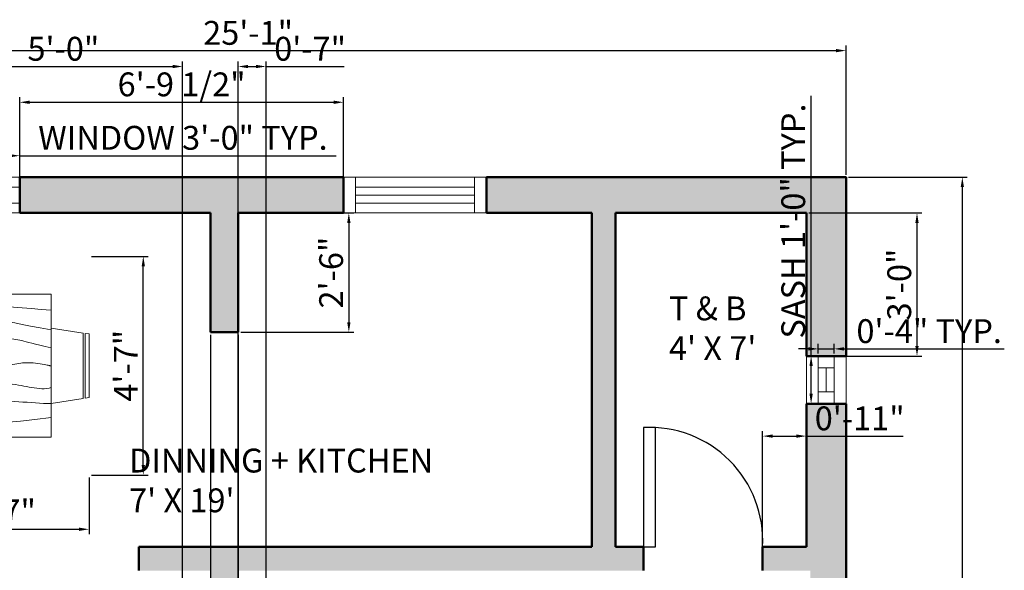
# Model space of a CAD drawing. Units: inches. Extents: x 2247 to 2697, y 1573 to 2133.
# Tile 4 of 4: x 2409 to 2657, y 1993 to 2132. Entities that reach past the tile are written whole.
import ezdxf

# ---------------------------------------------------------------- set-up
doc = ezdxf.new("R2010")
doc.units = ezdxf.units.IN
for name, color, linetype, lineweight in [('A-ANNO-DIMS', 2, 'Continuous', 18), ('A-AREA-IDEN', 7, 'Continuous', 25), ('A-DOOR', 4, 'Continuous', 25), ('A-FURN', 8, 'Continuous', 18), ('A-GLAZ', 4, 'Continuous', 18), ('A-WALL', 7, 'Continuous', 50)]:
    doc.layers.add(name, color=color, linetype=linetype, lineweight=lineweight)
doc.layers.add('A-WALL-PATT', color=67, linetype='Continuous', lineweight=13, true_color=0x727430)
doc.styles.get("Standard").update_dxf_attribs({"font": 'arial.ttf'})
doc.dimstyles.new('ISO-25', dxfattribs={"dimtxt": 6, "dimasz": 2.5, "dimexe": 1.25, "dimexo": 0.625, "dimtad": 1, "dimlunit": 3, "dimtxsty": 'Standard', "dimcen": 2.5, "dimadec": 0, "dimazin": 0, "dimtfac": 1, "dimtmove": 0, "dimatfit": 3, "dimfxl": 1, "dimarcsym": 0})

# ---------------------------------------------------------------- blocks, each defined once
blk = doc.blocks.new('*D1')
at = {"layer": 'A-ANNO-DIMS', "color": 0, "lineweight": -2, "transparency": 16777216}
for p, q in [((2316.09, 2092.98), (2316.09, 2125.46)), ((2318.59, 2124.21), (2614.59, 2124.21)), ((2617.09, 2092.98), (2617.09, 2125.46))]:
    blk.add_line(p, q, dxfattribs=at)
at = {"layer": 'A-ANNO-DIMS', "color": 0, "transparency": 16777216}
for points in [[(2318.59, 2124.63), (2318.59, 2123.79), (2316.09, 2124.21)], [(2614.59, 2124.63), (2614.59, 2123.79), (2617.09, 2124.21)]]:
    blk.add_solid(points, dxfattribs=at)
at = {"layer": 'Defpoints', "color": 0, "transparency": 16777216}
for p in [(2617.09, 2124.21), (2316.09, 2092.36), (2617.09, 2092.36)]:
    blk.add_point(p, dxfattribs=at)
at = {"layer": 'A-ANNO-DIMS', "color": 0, "transparency": 16777216, "insert": (2466.59, 2127.9), "char_height": 6, "attachment_point": 5}
blk.add_mtext('25\'-1"', dxfattribs=at)
blk = doc.blocks.new('*D2')
at = {"layer": 'A-ANNO-DIMS', "color": 0, "lineweight": -2, "transparency": 16777216}
for p, q in [((2617.72, 2092.36), (2647.6, 2092.36)), ((2646.35, 2089.86), (2646.35, 1604.86)), ((2617.72, 1602.36), (2647.6, 1602.36))]:
    blk.add_line(p, q, dxfattribs=at)
at = {"layer": 'A-ANNO-DIMS', "color": 0, "transparency": 16777216}
for points in [[(2645.94, 2089.86), (2646.77, 2089.86), (2646.35, 2092.36)], [(2645.94, 1604.86), (2646.77, 1604.86), (2646.35, 1602.36)]]:
    blk.add_solid(points, dxfattribs=at)
at = {"layer": 'Defpoints', "color": 0, "transparency": 16777216}
for p in [(2617.09, 2092.36), (2617.09, 1602.36), (2646.35, 1602.36)]:
    blk.add_point(p, dxfattribs=at)
at = {"layer": 'A-ANNO-DIMS', "color": 0, "transparency": 16777216, "insert": (2642.66, 1847.36), "char_height": 6, "attachment_point": 5, "rotation": 90}
blk.add_mtext('40\'-10"', dxfattribs=at)
blk = doc.blocks.new('Dining Set - 36 x 72 in.')
for p, q in [((-22, 27.5), (-22.1562, 26.50042)), ((-22, 27.5), (-6, 27.5)), ((-5.8437, 26.49966), (-6, 27.5)), ((6, 27.5), (5.8438, 26.50042)), ((6, 27.5), (22, 27.5)), ((22.1563, 26.49966), (22, 27.5)), ((-22.2343, 26.00059), (-23.4847, 17.99762)), ((-22.2304, 26), (-5.7608, 26)), ((-5.8416, 26.5), (-22.1534, 26.5)), ((-4.5152, 17.99762), (-5.7655, 25.99926)), ((5.7657, 26.00059), (4.5153, 17.99762)), ((5.7696, 26), (22.2392, 26)), ((22.1584, 26.5), (5.8466, 26.5)), ((23.4848, 17.99762), (22.2345, 25.99926)), ((36, 18), (-36, 18)), ((-36, 18), (-36, -18)), ((36, -18), (36, 18)), ((-45.5, 8), (-44.5004, 8.15617)), ((-45.5, 8), (-45.5, -8)), ((-44.5, -8.15843), (-44.5, 8.15338)), ((-44.0006, 8.23428), (-35.9976, 9.48474)), ((-44, 8.23041), (-44, -8.23915)), ((44.0006, 8.23428), (35.9976, 9.48474)), ((44, 8.23041), (44, -8.23915)), ((44.5, -8.15843), (44.5, 8.15338)), ((45.5, 8), (44.5005, 8.15617)), ((45.5, 8), (45.5, -8)), ((-44.4997, -8.15631), (-45.5, -8)), ((-35.9976, -9.48476), (-43.9993, -8.2345)), ((35.9976, -9.48476), (43.9993, -8.2345)), ((44.4997, -8.15631), (45.5, -8)), ((-36, -18), (36, -18)), ((-22.2343, -26.0006), (-23.4847, -17.99762)), ((-4.5152, -17.99762), (-5.7655, -25.99928)), ((5.7657, -26.0006), (4.5153, -17.99762)), ((23.4848, -17.99762), (22.2345, -25.99928)), ((-22.2304, -26), (-5.7608, -26)), ((-22, -27.5), (-22.1562, -26.50044)), ((-5.8416, -26.5), (-22.1534, -26.5)), ((-5.8437, -26.49967), (-6, -27.5)), ((5.7696, -26), (22.2392, -26)), ((6, -27.5), (5.8438, -26.50044)), ((22.1584, -26.5), (5.8466, -26.5)), ((22.1563, -26.49967), (22, -27.5)), ((-22, -27.5), (-6, -27.5)), ((6, -27.5), (22, -27.5))]:
    blk.add_line(p, q)
for points in [[(-36, 15), (-31.1772, 14.97754), (-26.8079, 14.91406), (-22.8538, 14.81543), (-19.276, 14.6875), (-16.0362, 14.53613), (-13.0957, 14.36718), (-10.4159, 14.18652), (-7.9583, 14), (-5.6904, 13.81315), (-3.6035, 13.63021), (-1.6954, 13.45508), (0.0365, 13.29166), (1.5945, 13.14388), (2.9811, 13.01562), (4.1988, 12.9108), (5.25, 12.83333), (6.1393, 12.78613), (6.8802, 12.76823), (7.4883, 12.77767), (7.9792, 12.8125), (8.3685, 12.87077), (8.6719, 12.95052), (8.9049, 13.0498), (9.0833, 13.16666), (9.2205, 13.29899), (9.3216, 13.44401), (9.3895, 13.59879), (9.4271, 13.76041), (9.4373, 13.92594), (9.4232, 14.09245), (9.3875, 14.257), (9.3333, 14.41666), (9.2638, 14.56917), (9.1836, 14.71484), (9.0975, 14.85465), (9.0104, 14.98958), (8.9272, 15.1206), (8.8529, 15.2487), (8.7922, 15.37483), (8.75, 15.5), (8.7305, 15.62467), (8.7344, 15.74739), (8.7617, 15.86621), (8.8125, 15.97916), (8.8867, 16.08431), (8.9844, 16.17968), (9.1055, 16.26334), (9.25, 16.33333), (9.4189, 16.38802), (9.6172, 16.42708), (9.8506, 16.45052), (10.125, 16.45833), (10.4463, 16.45052), (10.8203, 16.42708), (11.2529, 16.38802), (11.75, 16.33333), (12.3184, 16.26318), (12.9694, 16.17838), (13.7151, 16.07991), (14.5677, 15.96875), (15.5395, 15.84586), (16.6426, 15.71224), (17.8893, 15.56884), (19.2917, 15.41666), (20.859, 15.25667), (22.5879, 15.08984), (24.4721, 14.91715), (26.5052, 14.73958), (28.6809, 14.5581), (30.9929, 14.3737), (33.4347, 14.18733), (36, 14)], [(-36, 10), (-28.9766, 10.14274), (-23.1725, 10.20442), (-18.4241, 10.19775), (-14.5677, 10.13541), (-11.4399, 10.03011), (-8.877, 9.89453), (-6.7154, 9.74137), (-4.7917, 9.58333), (-2.9698, 9.43082), (-1.2246, 9.28515), (0.4415, 9.14534), (2.026, 9.01041), (3.5266, 8.87939), (4.9408, 8.7513), (6.266, 8.62516), (7.5, 8.5), (8.6411, 8.37549), (9.6914, 8.2539), (10.6538, 8.13818), (11.5312, 8.03125), (12.3267, 7.93603), (13.043, 7.85547), (13.6831, 7.79248), (14.25, 7.75), (14.7471, 7.7303), (15.1797, 7.73307), (15.5537, 7.75732), (15.875, 7.80208), (16.1494, 7.86637), (16.3828, 7.94922), (16.5811, 8.04964), (16.75, 8.16666), (16.8944, 8.29915), (17.0143, 8.44531), (17.1089, 8.60319), (17.1771, 8.77083), (17.218, 8.94629), (17.2305, 9.1276), (17.2137, 9.31282), (17.1667, 9.5), (17.0895, 9.6875), (16.987, 9.875), (16.8649, 10.0625), (16.7292, 10.25), (16.5856, 10.4375), (16.4401, 10.625), (16.2985, 10.8125), (16.1667, 11), (16.05, 11.18733), (15.9518, 11.3737), (15.8752, 11.5581), (15.8229, 11.73958), (15.798, 11.91715), (15.8034, 12.08984), (15.842, 12.25667), (15.9167, 12.41666), (16.0295, 12.56836), (16.1784, 12.70833), (16.3605, 12.83268), (16.5729, 12.9375), (16.8127, 13.01888), (17.0768, 13.07291), (17.3625, 13.0957), (17.6667, 13.08333), (17.9894, 13.03312), (18.3418, 12.94726), (18.7382, 12.82918), (19.1927, 12.68229), (19.7195, 12.51001), (20.3327, 12.31575), (21.0465, 12.10294), (21.875, 11.875), (22.8357, 11.63354), (23.959, 11.37304), (25.2786, 11.08618), (26.8282, 10.76562), (28.6414, 10.40405), (30.752, 9.99414), (33.1936, 9.52856), (36, 9)], [(-36, 5.5), (-30.7157, 5.3348), (-26.069, 5.20963), (-21.9946, 5.11767), (-18.4271, 5.05208), (-15.3009, 5.00602), (-12.5508, 4.97265), (-10.1112, 4.94515), (-7.9167, 4.91666), (-5.909, 4.88167), (-4.0586, 4.83984), (-2.3429, 4.79215), (-0.7396, 4.73958), (0.7739, 4.6831), (2.22, 4.6237), (3.6213, 4.56233), (5, 4.5), (6.373, 4.43782), (7.7344, 4.3776), (9.0723, 4.32129), (10.375, 4.27083), (11.6309, 4.22819), (12.8281, 4.19531), (13.9551, 4.17415), (15, 4.16666), (15.954, 4.17448), (16.819, 4.19791), (17.6001, 4.23698), (18.3021, 4.29166), (18.9299, 4.36198), (19.4883, 4.44791), (19.9823, 4.54948), (20.4167, 4.66666), (20.7969, 4.79899), (21.1302, 4.94401), (21.4245, 5.09879), (21.6875, 5.26041), (21.9271, 5.42594), (22.1511, 5.59245), (22.3672, 5.757), (22.5834, 5.91666), (22.8065, 6.06868), (23.0404, 6.21093), (23.2879, 6.34147), (23.5521, 6.45833), (23.8358, 6.55957), (24.142, 6.64323), (24.4735, 6.70735), (24.8334, 6.75), (25.2235, 6.76969), (25.642, 6.76692), (26.0858, 6.74267), (26.5521, 6.69791), (27.0379, 6.63362), (27.5404, 6.55078), (28.0565, 6.45036), (28.5834, 6.33333), (29.1242, 6.19987), (29.7071, 6.04687), (30.3661, 5.87044), (31.1354, 5.66666), (32.0493, 5.43164), (33.142, 5.16146), (34.4475, 4.85221), (36, 4.5)], [(-36, -1), (-30.7915, -0.6591), (-26.0195, -0.38216), (-21.6519, -0.16284), (-17.6563, 0.00521), (-14.0005, 0.12833), (-10.6523, 0.21289), (-7.5796, 0.26522), (-4.75, 0.29166), (-2.134, 0.29793), (0.2878, 0.28711), (2.5317, 0.26163), (4.6146, 0.22396), (6.5529, 0.17651), (8.3633, 0.12174), (10.0623, 0.06209), (11.6667, 0), (13.1899, -0.06201), (14.6341, -0.1211), (15.9982, -0.17432), (17.2813, -0.21875), (18.4823, -0.25147), (19.6003, -0.26953), (20.6343, -0.27002), (21.5834, -0.25), (22.4481, -0.20768), (23.2357, -0.14584), (23.9549, -0.06836), (24.6146, 0.02083), (25.2235, 0.11784), (25.7904, 0.21875), (26.3241, 0.31966), (26.8334, 0.41666), (27.3265, 0.50618), (27.8099, 0.58593), (28.2894, 0.65397), (28.7709, 0.70833), (29.2601, 0.74707), (29.763, 0.76823), (30.2855, 0.76985), (30.8334, 0.75), (31.4088, 0.70784), (31.9994, 0.64713), (32.589, 0.57275), (33.1615, 0.48958), (33.7008, 0.4025), (34.1908, 0.3164), (34.6153, 0.23616), (34.9584, 0.16666), (35.2099, 0.11165), (35.3848, 0.07031), (35.504, 0.04069), (35.5886, 0.02083), (35.6594, 0.00879), (35.7377, 0.0026), (35.8442, 0.00032), (36, 0)], [(-36, -6.5), (-27.1843, -6.31267), (-20.084, -6.1263), (-14.469, -5.9419), (-10.1094, -5.76042), (-6.7752, -5.58285), (-4.2363, -5.41016), (-2.2629, -5.24333), (-0.625, -5.08334), (0.8708, -4.93099), (2.2715, -4.78646), (3.5872, -4.64974), (4.8281, -4.52084), (6.0046, -4.39974), (7.127, -4.28646), (8.2053, -4.18099), (9.25, -4.08334), (10.2705, -3.99382), (11.2734, -3.91407), (12.2647, -3.84603), (13.25, -3.79167), (14.2354, -3.75293), (15.2266, -3.73177), (16.2295, -3.73015), (17.25, -3.75), (18.2912, -3.79248), (19.3451, -3.85547), (20.4009, -3.93604), (21.4479, -4.03125), (22.4754, -4.13819), (23.4727, -4.25391), (24.4289, -4.37549), (25.3334, -4.5), (26.1785, -4.62492), (26.9694, -4.74935), (27.7145, -4.87281), (28.4219, -4.99479), (29.1, -5.11483), (29.7572, -5.23242), (30.4016, -5.34709), (31.0417, -5.45834), (31.6837, -5.56437), (32.3262, -5.65821), (32.9658, -5.73153), (33.599, -5.77604), (34.2224, -5.78345), (34.8327, -5.74545), (35.4264, -5.65373), (36, -5.5)], [(-36, -10), (-26.4022, -9.81299), (-18.4675, -9.62891), (-11.9839, -9.45069), (-6.7396, -9.28125), (-2.5226, -9.12354), (0.8789, -8.98047), (3.6769, -8.85498), (6.0833, -8.75), (8.2767, -8.66765), (10.3021, -8.60677), (12.1712, -8.56543), (13.8958, -8.54167), (15.4876, -8.53353), (16.9583, -8.53907), (18.3197, -8.55632), (19.5834, -8.58334), (20.7616, -8.61841), (21.8685, -8.66081), (22.9188, -8.71004), (23.9271, -8.76563), (24.9081, -8.82707), (25.8763, -8.89388), (26.8465, -8.96558), (27.8334, -9.04167), (28.8474, -9.12118), (29.8828, -9.20117), (30.93, -9.27824), (31.9792, -9.34896), (33.0205, -9.40991), (34.0443, -9.45768), (35.0407, -9.48885), (36, -9.5)], [(-36, -14.5), (-30.0881, -14.33513), (-25.0332, -14.21224), (-20.7312, -14.12647), (-17.0781, -14.07292), (-13.97, -14.04671), (-11.3027, -14.04297), (-8.9724, -14.05681), (-6.875, -14.08334), (-4.9224, -14.11833), (-3.0905, -14.16016), (-1.3709, -14.20785), (0.2448, -14.26042), (1.7647, -14.3169), (3.1973, -14.3763), (4.5507, -14.43767), (5.8333, -14.5), (7.0554, -14.5621), (8.235, -14.62175), (9.3922, -14.67652), (10.5469, -14.72396), (11.7192, -14.76164), (12.929, -14.78711), (14.1965, -14.79794), (15.5417, -14.79167), (16.9933, -14.76424), (18.6152, -14.70508), (20.4804, -14.60197), (22.6615, -14.44271), (25.2312, -14.21509), (28.2624, -13.9069), (31.8277, -13.50594), (36, -13)]]:
    blk.add_lwpolyline(points)
blk = doc.blocks.new('DOOR-SWING-30IN')
blk.add_lwpolyline([(0, 0), (3, 0), (3, 30), (0, 30)], close=True)
blk.add_arc((1.5, 1.5), 28.54, 356.9872, 93.0128)
blk = doc.blocks.new('WIN-36IN')
for p, q in [((0, 9), (36, 9)), ((0, 6.5), (36, 6.5)), ((3, 2.5), (3, 6.5)), ((33, 2.5), (33, 6.5)), ((0, 2.5), (36, 2.5)), ((3, 4.5), (33, 4.5)), ((0, 0), (36, 0))]:
    blk.add_line(p, q)
blk = doc.blocks.new('WIN-SASH-12IN')
for p, q in [((0, 0), (0, 12)), ((4, 0), (4, 12)), ((0, 9), (4, 9)), ((2, 3), (2, 9)), ((0, 3), (4, 3))]:
    blk.add_line(p, q)
blk = doc.blocks.new('*D13')
at = {"layer": 'A-ANNO-DIMS', "color": 0, "lineweight": -2, "transparency": 16777216}
for p, q in [((2373.09, 2092.98), (2373.09, 2099.01)), ((2375.59, 2097.76), (2406.59, 2097.76)), ((2409.09, 2092.98), (2409.09, 2099.01)), ((2409.09, 2097.76), (2488.77, 2097.76))]:
    blk.add_line(p, q, dxfattribs=at)
at = {"layer": 'A-ANNO-DIMS', "color": 0, "transparency": 16777216}
for points in [[(2375.59, 2098.18), (2375.59, 2097.34), (2373.09, 2097.76)], [(2406.59, 2098.18), (2406.59, 2097.34), (2409.09, 2097.76)]]:
    blk.add_solid(points, dxfattribs=at)
at = {"layer": 'Defpoints', "color": 0, "transparency": 16777216}
for p in [(2409.09, 2097.76), (2373.09, 2092.36), (2409.09, 2092.36)]:
    blk.add_point(p, dxfattribs=at)
at = {"layer": 'A-ANNO-DIMS', "color": 0, "transparency": 16777216, "insert": (2450.18, 2101.49), "char_height": 6, "attachment_point": 5}
blk.add_mtext('WINDOW 3\'-0" TYP.', dxfattribs=at)
blk = doc.blocks.new('*D17')
at = {"layer": 'A-ANNO-DIMS', "color": 0, "lineweight": -2, "transparency": 16777216}
for p, q in [((2608.29, 2047.36), (2608.29, 2112.81)), ((2609.47, 2047.36), (2607.04, 2047.36)), ((2608.29, 2037.86), (2608.29, 2044.86)), ((2609.47, 2035.36), (2607.04, 2035.36))]:
    blk.add_line(p, q, dxfattribs=at)
at = {"layer": 'A-ANNO-DIMS', "color": 0, "transparency": 16777216}
for points in [[(2607.88, 2044.86), (2608.71, 2044.86), (2608.29, 2047.36)], [(2607.88, 2037.86), (2608.71, 2037.86), (2608.29, 2035.36)]]:
    blk.add_solid(points, dxfattribs=at)
at = {"layer": 'Defpoints', "color": 0, "transparency": 16777216}
for p in [(2608.29, 2047.36), (2610.09, 2047.36), (2610.09, 2035.36)]:
    blk.add_point(p, dxfattribs=at)
at = {"layer": 'A-ANNO-DIMS', "color": 0, "transparency": 16777216, "insert": (2604.57, 2081.33), "char_height": 6, "attachment_point": 5, "rotation": 90}
blk.add_mtext('SASH 1\'-0" TYP.', dxfattribs=at)
blk = doc.blocks.new('*D18')
at = {"layer": 'A-ANNO-DIMS', "color": 0, "lineweight": -2, "transparency": 16777216}
for p, q in [((2610.09, 2047.98), (2610.09, 2050.41)), ((2614.09, 2047.98), (2614.09, 2050.41)), ((2607.59, 2049.16), (2605.09, 2049.16)), ((2610.09, 2049.16), (2614.09, 2049.16)), ((2616.59, 2049.16), (2656.92, 2049.16))]:
    blk.add_line(p, q, dxfattribs=at)
at = {"layer": 'A-ANNO-DIMS', "color": 0, "transparency": 16777216}
for points in [[(2607.59, 2049.58), (2607.59, 2048.74), (2610.09, 2049.16)], [(2616.59, 2049.58), (2616.59, 2048.74), (2614.09, 2049.16)]]:
    blk.add_solid(points, dxfattribs=at)
at = {"layer": 'Defpoints', "color": 0, "transparency": 16777216}
for p in [(2610.09, 2047.36), (2614.09, 2049.16), (2614.09, 2047.36)]:
    blk.add_point(p, dxfattribs=at)
at = {"layer": 'A-ANNO-DIMS', "color": 0, "transparency": 16777216, "insert": (2638.01, 2052.85), "char_height": 6, "attachment_point": 5}
blk.add_mtext('0\'-4" TYP.', dxfattribs=at)
blk = doc.blocks.new('*D21')
at = {"layer": 'A-ANNO-DIMS', "color": 0, "lineweight": -2, "transparency": 16777216}
for p, q in [((2335.55, 2016.79), (2335.55, 2002.52)), ((2426.55, 2016.79), (2426.55, 2002.52)), ((2338.05, 2003.77), (2424.05, 2003.77))]:
    blk.add_line(p, q, dxfattribs=at)
at = {"layer": 'A-ANNO-DIMS', "color": 0, "transparency": 16777216}
for points in [[(2338.05, 2004.18), (2338.05, 2003.35), (2335.55, 2003.77)], [(2424.05, 2004.18), (2424.05, 2003.35), (2426.55, 2003.77)]]:
    blk.add_solid(points, dxfattribs=at)
at = {"layer": 'Defpoints', "color": 0, "transparency": 16777216}
for p in [(2335.55, 2017.42), (2426.55, 2017.42), (2426.55, 2003.77)]:
    blk.add_point(p, dxfattribs=at)
at = {"layer": 'A-ANNO-DIMS', "color": 0, "transparency": 16777216, "insert": (2381.05, 2007.49), "char_height": 6, "attachment_point": 5}
blk.add_mtext('DINING SET 7\'-7"', dxfattribs=at)
blk = doc.blocks.new('*D22')
at = {"layer": 'A-ANNO-DIMS', "color": 0, "lineweight": -2, "transparency": 16777216}
for p, q in [((2427.18, 2072.42), (2441.45, 2072.42)), ((2440.2, 2019.92), (2440.2, 2069.92)), ((2427.18, 2017.42), (2441.45, 2017.42))]:
    blk.add_line(p, q, dxfattribs=at)
at = {"layer": 'A-ANNO-DIMS', "color": 0, "transparency": 16777216}
for points in [[(2439.79, 2069.92), (2440.62, 2069.92), (2440.2, 2072.42)], [(2439.79, 2019.92), (2440.62, 2019.92), (2440.2, 2017.42)]]:
    blk.add_solid(points, dxfattribs=at)
at = {"layer": 'Defpoints', "color": 0, "transparency": 16777216}
for p in [(2426.55, 2072.42), (2440.2, 2072.42), (2426.55, 2017.42)]:
    blk.add_point(p, dxfattribs=at)
at = {"layer": 'A-ANNO-DIMS', "color": 0, "transparency": 16777216, "insert": (2436.58, 2044.92), "char_height": 6, "attachment_point": 5, "rotation": 90}
blk.add_mtext('4\'-7"', dxfattribs=at)
blk = doc.blocks.new('*D24')
at = {"layer": 'A-ANNO-DIMS', "color": 0, "lineweight": -2, "transparency": 16777216}
for p, q in [((2409.09, 2083.98), (2409.09, 2112.46)), ((2490.59, 2083.98), (2490.59, 2112.46)), ((2411.59, 2111.21), (2488.09, 2111.21))]:
    blk.add_line(p, q, dxfattribs=at)
at = {"layer": 'A-ANNO-DIMS', "color": 0, "transparency": 16777216}
for points in [[(2411.59, 2111.63), (2411.59, 2110.79), (2409.09, 2111.21)], [(2488.09, 2111.63), (2488.09, 2110.79), (2490.59, 2111.21)]]:
    blk.add_solid(points, dxfattribs=at)
at = {"layer": 'Defpoints', "color": 0, "transparency": 16777216}
for p in [(2490.59, 2111.21), (2409.09, 2083.36), (2490.59, 2083.36)]:
    blk.add_point(p, dxfattribs=at)
at = {"layer": 'A-ANNO-DIMS', "color": 0, "transparency": 16777216, "insert": (2449.84, 2114.94), "char_height": 6, "attachment_point": 5}
blk.add_mtext('6\'-9 1/2"', dxfattribs=at)
blk = doc.blocks.new('*D25')
at = {"layer": 'A-ANNO-DIMS', "color": 0, "lineweight": -2, "transparency": 16777216}
for p, q in [((2464.72, 2083.36), (2493.19, 2083.36)), ((2491.94, 2080.86), (2491.94, 2055.86)), ((2464.72, 2053.36), (2493.19, 2053.36))]:
    blk.add_line(p, q, dxfattribs=at)
at = {"layer": 'A-ANNO-DIMS', "color": 0, "transparency": 16777216}
for points in [[(2491.53, 2080.86), (2492.36, 2080.86), (2491.94, 2083.36)], [(2491.53, 2055.86), (2492.36, 2055.86), (2491.94, 2053.36)]]:
    blk.add_solid(points, dxfattribs=at)
at = {"layer": 'Defpoints', "color": 0, "transparency": 16777216}
for p in [(2464.09, 2083.36), (2464.09, 2053.36), (2491.94, 2053.36)]:
    blk.add_point(p, dxfattribs=at)
at = {"layer": 'A-ANNO-DIMS', "color": 0, "transparency": 16777216, "insert": (2488.26, 2068.36), "char_height": 6, "attachment_point": 5, "rotation": 90}
blk.add_mtext('2\'-6"', dxfattribs=at)
blk = doc.blocks.new('*D26')
at = {"layer": 'A-ANNO-DIMS', "color": 0, "lineweight": -2, "transparency": 16777216}
for p, q in [((2457.09, 2052.73), (2457.09, 1573.26)), ((2464.09, 2052.73), (2464.09, 1573.26)), ((2459.59, 1574.51), (2461.59, 1574.51)), ((2464.09, 1574.51), (2483.79, 1574.51))]:
    blk.add_line(p, q, dxfattribs=at)
at = {"layer": 'A-ANNO-DIMS', "color": 0, "transparency": 16777216}
for points in [[(2459.59, 1574.93), (2459.59, 1574.09), (2457.09, 1574.51)], [(2461.59, 1574.93), (2461.59, 1574.09), (2464.09, 1574.51)]]:
    blk.add_solid(points, dxfattribs=at)
at = {"layer": 'Defpoints', "color": 0, "transparency": 16777216}
for p in [(2457.09, 2053.36), (2464.09, 2053.36), (2464.09, 1574.51)]:
    blk.add_point(p, dxfattribs=at)
at = {"layer": 'A-ANNO-DIMS', "color": 0, "transparency": 16777216, "insert": (2475.19, 1578.2), "char_height": 6, "attachment_point": 5}
blk.add_mtext('0\'-7"', dxfattribs=at)
blk = doc.blocks.new('*D27')
at = {"layer": 'A-ANNO-DIMS', "color": 0, "lineweight": -2, "transparency": 16777216}
for p, q in [((2607.72, 2083.36), (2636.19, 2083.36)), ((2634.94, 2080.86), (2634.94, 2049.86)), ((2607.72, 2047.36), (2636.19, 2047.36))]:
    blk.add_line(p, q, dxfattribs=at)
at = {"layer": 'A-ANNO-DIMS', "color": 0, "transparency": 16777216}
for points in [[(2634.53, 2080.86), (2635.36, 2080.86), (2634.94, 2083.36)], [(2634.53, 2049.86), (2635.36, 2049.86), (2634.94, 2047.36)]]:
    blk.add_solid(points, dxfattribs=at)
at = {"layer": 'Defpoints', "color": 0, "transparency": 16777216}
for p in [(2607.09, 2083.36), (2607.09, 2047.36), (2634.94, 2047.36)]:
    blk.add_point(p, dxfattribs=at)
at = {"layer": 'A-ANNO-DIMS', "color": 0, "transparency": 16777216, "insert": (2631.25, 2065.36), "char_height": 6, "attachment_point": 5, "rotation": 90}
blk.add_mtext('3\'-0"', dxfattribs=at)
blk = doc.blocks.new('*D38')
at = {"layer": 'A-ANNO-DIMS', "color": 0, "lineweight": -2, "transparency": 16777216}
for p, q in [((2390.09, 1693.98), (2390.09, 2121.46)), ((2450.09, 1693.98), (2450.09, 2121.46)), ((2392.59, 2120.21), (2447.59, 2120.21))]:
    blk.add_line(p, q, dxfattribs=at)
at = {"layer": 'A-ANNO-DIMS', "color": 0, "transparency": 16777216}
for points in [[(2392.59, 2120.63), (2392.59, 2119.79), (2390.09, 2120.21)], [(2447.59, 2120.63), (2447.59, 2119.79), (2450.09, 2120.21)]]:
    blk.add_solid(points, dxfattribs=at)
at = {"layer": 'Defpoints', "color": 0, "transparency": 16777216}
for p in [(2450.09, 2120.21), (2390.09, 1693.36), (2450.09, 1693.36)]:
    blk.add_point(p, dxfattribs=at)
at = {"layer": 'A-ANNO-DIMS', "color": 0, "transparency": 16777216, "insert": (2420.09, 2123.9), "char_height": 6, "attachment_point": 5}
blk.add_mtext('5\'-0"', dxfattribs=at)
blk = doc.blocks.new('*D42')
at = {"layer": 'A-ANNO-DIMS', "color": 0, "lineweight": -2, "transparency": 16777216}
for p, q in [((2464.09, 1873.98), (2464.09, 2121.46)), ((2471.09, 1873.98), (2471.09, 2121.46)), ((2466.59, 2120.21), (2468.59, 2120.21)), ((2471.09, 2120.21), (2490.79, 2120.21))]:
    blk.add_line(p, q, dxfattribs=at)
at = {"layer": 'A-ANNO-DIMS', "color": 0, "transparency": 16777216}
for points in [[(2466.59, 2120.63), (2466.59, 2119.79), (2464.09, 2120.21)], [(2468.59, 2120.63), (2468.59, 2119.79), (2471.09, 2120.21)]]:
    blk.add_solid(points, dxfattribs=at)
at = {"layer": 'Defpoints', "color": 0, "transparency": 16777216}
for p in [(2471.09, 2120.21), (2464.09, 1873.36), (2471.09, 1873.36)]:
    blk.add_point(p, dxfattribs=at)
at = {"layer": 'A-ANNO-DIMS', "color": 0, "transparency": 16777216, "insert": (2482.19, 2123.9), "char_height": 6, "attachment_point": 5}
blk.add_mtext('0\'-7"', dxfattribs=at)
blk = doc.blocks.new('*D43')
at = {"layer": 'A-ANNO-DIMS', "color": 0, "lineweight": -2, "transparency": 16777216}
for p, q in [((2596.09, 1999.98), (2596.09, 2028.46)), ((2598.59, 2027.21), (2604.59, 2027.21)), ((2607.09, 1999.98), (2607.09, 2028.46)), ((2607.09, 2027.21), (2631.46, 2027.21))]:
    blk.add_line(p, q, dxfattribs=at)
at = {"layer": 'A-ANNO-DIMS', "color": 0, "transparency": 16777216}
for points in [[(2598.59, 2027.63), (2598.59, 2026.79), (2596.09, 2027.21)], [(2604.59, 2027.63), (2604.59, 2026.79), (2607.09, 2027.21)]]:
    blk.add_solid(points, dxfattribs=at)
at = {"layer": 'Defpoints', "color": 0, "transparency": 16777216}
for p in [(2607.09, 2027.21), (2596.09, 1999.36), (2607.09, 1999.36)]:
    blk.add_point(p, dxfattribs=at)
at = {"layer": 'A-ANNO-DIMS', "color": 0, "transparency": 16777216, "insert": (2620.52, 2030.9), "char_height": 6, "attachment_point": 5}
blk.add_mtext('0\'-11"', dxfattribs=at)

msp = doc.modelspace()

# ---------------------------------------------------------------- hatches: boundary and pattern name
at = {"layer": 'A-WALL-PATT'}
h = msp.add_hatch(color=256, dxfattribs=at)
h.dxf.hatch_style = 1
h.paths.add_polyline_path([(2490.594, 2092.36), (2409.094, 2092.36), (2409.094, 2083.36), (2457.094, 2083.36), (2457.094, 2053.36), (2464.094, 2053.36), (2464.094, 2083.36), (2490.594, 2083.36)])
h = msp.add_hatch(color=256, dxfattribs=at)
h.dxf.hatch_style = 1
h.paths.add_polyline_path([(2566.094, 1999.36), (2559.094, 1999.36), (2559.094, 2083.36), (2607.094, 2083.36), (2607.094, 2047.36), (2617.094, 2047.36), (2617.094, 2092.36), (2526.594, 2092.36), (2526.594, 2083.36), (2553.094, 2083.36), (2553.094, 1999.36), (2464.094, 1999.36), (2439.094, 1999.36), (2439.094, 1993.36), (2457.094, 1993.36), (2457.094, 1867.36), (2471.094, 1867.36), (2471.094, 1873.36), (2464.094, 1873.36), (2464.094, 1993.36), (2566.094, 1993.36)])
h = msp.add_hatch(color=256, dxfattribs=at)
h.dxf.hatch_style = 1
h.paths.add_polyline_path([(2617.094, 2035.36), (2607.094, 2035.36), (2607.094, 1999.36), (2596.094, 1999.36), (2596.094, 1993.36), (2608.094, 1993.36), (2608.094, 1951.36), (2617.094, 1951.36)])

# ---------------------------------------------------------------- linework, layer by layer
at = {"layer": 'A-GLAZ'}
for p, q in [((2490.594, 2092.36), (2506.991, 2092.36)), ((2493.594, 2083.36), (2493.594, 2092.36)), ((2506.991, 2092.36), (2526.594, 2092.36)), ((2523.594, 2083.36), (2523.594, 2092.36)), ((2493.594, 2089.86), (2523.594, 2089.86)), ((2493.594, 2087.86), (2523.594, 2087.86)), ((2493.594, 2085.86), (2523.594, 2085.86)), ((2526.594, 2083.36), (2490.594, 2083.36)), ((2607.094, 2047.36), (2607.094, 2035.36)), ((2617.094, 2047.36), (2617.094, 2035.36))]:
    msp.add_line(p, q, dxfattribs=at)
at = {"layer": 'A-WALL'}
for p, q in [((2409.094, 2083.36), (2409.094, 2092.36)), ((2490.594, 2083.36), (2490.594, 2092.36)), ((2526.594, 2083.36), (2526.594, 2092.36)), ((2409.094, 2083.36), (2457.094, 2083.36)), ((2457.094, 2053.36), (2457.094, 2083.36)), ((2464.094, 2053.36), (2464.094, 2083.36)), ((2464.094, 2083.36), (2490.594, 2083.36)), ((2526.594, 2083.36), (2553.094, 2083.36)), ((2553.094, 1999.36), (2553.094, 2083.36)), ((2559.094, 1999.36), (2559.094, 2083.36)), ((2559.094, 2083.36), (2607.094, 2083.36)), ((2607.094, 2083.36), (2607.094, 2047.36)), ((2457.094, 2053.36), (2464.094, 2053.36)), ((2607.094, 2047.36), (2617.094, 2047.36)), ((2607.094, 2035.36), (2617.094, 2035.36)), ((2607.094, 2035.36), (2607.094, 1999.36)), ((2439.094, 1993.36), (2439.094, 1999.36)), ((2439.094, 1999.36), (2464.094, 1999.36)), ((2464.094, 1999.36), (2553.094, 1999.36)), ((2559.094, 1999.36), (2566.094, 1999.36)), ((2566.094, 1999.36), (2566.094, 1993.36)), ((2596.094, 1999.36), (2596.094, 1993.36)), ((2596.094, 1999.36), (2607.094, 1999.36))]:
    msp.add_line(p, q, dxfattribs=at)
for points in [[(2409.094, 2092.36), (2490.594, 2092.36)], [(2526.594, 2092.36), (2617.094, 2092.36), (2617.094, 2047.36)], [(2617.094, 2035.36), (2617.094, 1951.36)]]:
    msp.add_lwpolyline(points, dxfattribs=at)

# ---------------------------------------------------------------- block references
at = {"layer": 'A-DOOR'}
msp.add_blockref('DOOR-SWING-30IN', (2566.094, 1999.36), dxfattribs=at)
at = {"layer": 'A-FURN'}
msp.add_blockref('Dining Set - 36 x 72 in.', (2381.053, 2044.916), dxfattribs=at)
at = {"layer": 'A-GLAZ'}
for name, p in [('WIN-36IN', (2373.094, 2083.36)), ('WIN-SASH-12IN', (2610.094, 2035.36))]:
    msp.add_blockref(name, p, dxfattribs=at)

# ---------------------------------------------------------------- texts
at = {"layer": 'A-AREA-IDEN', "char_height": 6, "attachment_point": 1}
for s, width, insert in [("T & B \\P4' X 7'", 23.42902, (2572.513, 2062.343)), ("DINNING + KITCHEN \\P7' X 19'", 90.99191, (2436.629, 2024.055))]:
    msp.add_mtext_dynamic_manual_height_columns(s, width=width, gutter_width=12.5, heights=[0], dxfattribs=dict(at, insert=insert))

# ---------------------------------------------------------------- dimensions: what is measured, and where the dimension line sits
at = {"layer": 'A-ANNO-DIMS'}
for base, p1, p2, override, picture, middle in [((2617.094, 2124.211), (2316.094, 2092.36), (2617.094, 2092.36), {"dimclrd": 0, "dimclre": 0, "dimclrt": 0}, '*D1', (2466.594, 2127.899)), ((2450.094, 2120.21), (2390.094, 1693.36), (2450.094, 1693.36), {"dimdec": 1, "dimlfac": 1, "dimrnd": 0, "dimzin": 1, "dimdsep": 46, "dimlunit": 4, "dimfrac": 2}, '*D38', (2420.094, 2123.898)), ((2471.094, 2120.21), (2464.094, 1873.36), (2471.094, 1873.36), {"dimdec": 1, "dimlfac": 1, "dimrnd": 0, "dimzin": 1, "dimdsep": 46, "dimlunit": 4, "dimfrac": 2}, '*D42', (2482.194, 2123.898)), ((2490.594, 2111.21), (2409.094, 2083.36), (2490.594, 2083.36), {"dimdec": 1, "dimlfac": 1, "dimrnd": 0, "dimzin": 1, "dimdsep": 46, "dimlunit": 4, "dimfrac": 2}, '*D24', (2449.844, 2114.937)), ((2464.094, 1574.51), (2457.094, 2053.36), (2464.094, 2053.36), {"dimdec": 1, "dimlfac": 1, "dimrnd": 0, "dimzin": 1, "dimdsep": 46, "dimlunit": 4, "dimfrac": 2}, '*D26', (2475.194, 1578.198)), ((2607.094, 2027.21), (2596.094, 1999.36), (2607.094, 1999.36), {"dimdec": 1, "dimlfac": 1, "dimrnd": 0, "dimzin": 1, "dimdsep": 46, "dimlunit": 4, "dimfrac": 2}, '*D43', (2620.525, 2030.898))]:
    dim = msp.add_linear_dim(base=base, p1=p1, p2=p2, dimstyle='ISO-25', override=override, dxfattribs=at)
    dim.commit()
    dim.dimension.update_dxf_attribs({"geometry": picture, "text_midpoint": middle})
for base, p1, p2, text, picture, middle in [((2409.094, 2097.76), (2373.094, 2092.36), (2409.094, 2092.36), 'WINDOW <> TYP.', '*D13', (2450.182, 2101.491)), ((2614.094, 2049.16), (2610.094, 2047.36), (2614.094, 2047.36), '<> TYP.', '*D18', (2638.006, 2052.848)), ((2426.553, 2003.766), (2335.553, 2017.416), (2426.553, 2017.416), 'DINING SET <>', '*D21', (2381.053, 2007.493))]:
    dim = msp.add_linear_dim(base=base, p1=p1, p2=p2, text=text, dimstyle='ISO-25', override={"dimdec": 1, "dimlfac": 1, "dimrnd": 0, "dimzin": 1, "dimdsep": 46, "dimlunit": 4, "dimfrac": 2}, dxfattribs=at)
    dim.commit()
    dim.dimension.update_dxf_attribs({"geometry": picture, "text_midpoint": middle})
dim = msp.add_linear_dim(base=(2608.294, 2047.36), p1=(2610.094, 2035.36), p2=(2610.094, 2047.36), angle=90, text='SASH <> TYP.', dimstyle='ISO-25', override={"dimdec": 1, "dimlfac": 1, "dimrnd": 0, "dimzin": 1, "dimdsep": 46, "dimlunit": 4, "dimfrac": 2}, dxfattribs=at)
dim.commit()
dim.dimension.update_dxf_attribs({"geometry": '*D17', "text_midpoint": (2604.567, 2081.334)})
for base, p1, p2, angle, override, picture, middle in [((2646.352, 1602.36), (2617.094, 2092.36), (2617.094, 1602.36), 90, {"dimclrd": 0, "dimclre": 0, "dimclrt": 0}, '*D2', (2642.664, 1847.36)), ((2491.944, 2053.36), (2464.094, 2083.36), (2464.094, 2053.36), 270, {"dimdec": 1, "dimlfac": 1, "dimrnd": 0, "dimzin": 1, "dimdsep": 46, "dimlunit": 4, "dimfrac": 2}, '*D25', (2488.256, 2068.36)), ((2634.944, 2047.36), (2607.094, 2083.36), (2607.094, 2047.36), 270, {"dimdec": 1, "dimlfac": 1, "dimrnd": 0, "dimzin": 1, "dimdsep": 46, "dimlunit": 4, "dimfrac": 2}, '*D27', (2631.254, 2065.36)), ((2440.203, 2072.416), (2426.553, 2017.416), (2426.553, 2072.416), 90, {"dimdec": 1, "dimlfac": 1, "dimrnd": 0, "dimzin": 1, "dimdsep": 46, "dimlunit": 4, "dimfrac": 2}, '*D22', (2436.578, 2044.916))]:
    dim = msp.add_linear_dim(base=base, p1=p1, p2=p2, angle=angle, dimstyle='ISO-25', override=override, dxfattribs=at)
    dim.commit()
    dim.dimension.update_dxf_attribs({"geometry": picture, "text_midpoint": middle})

doc.saveas('drawing.dxf')
